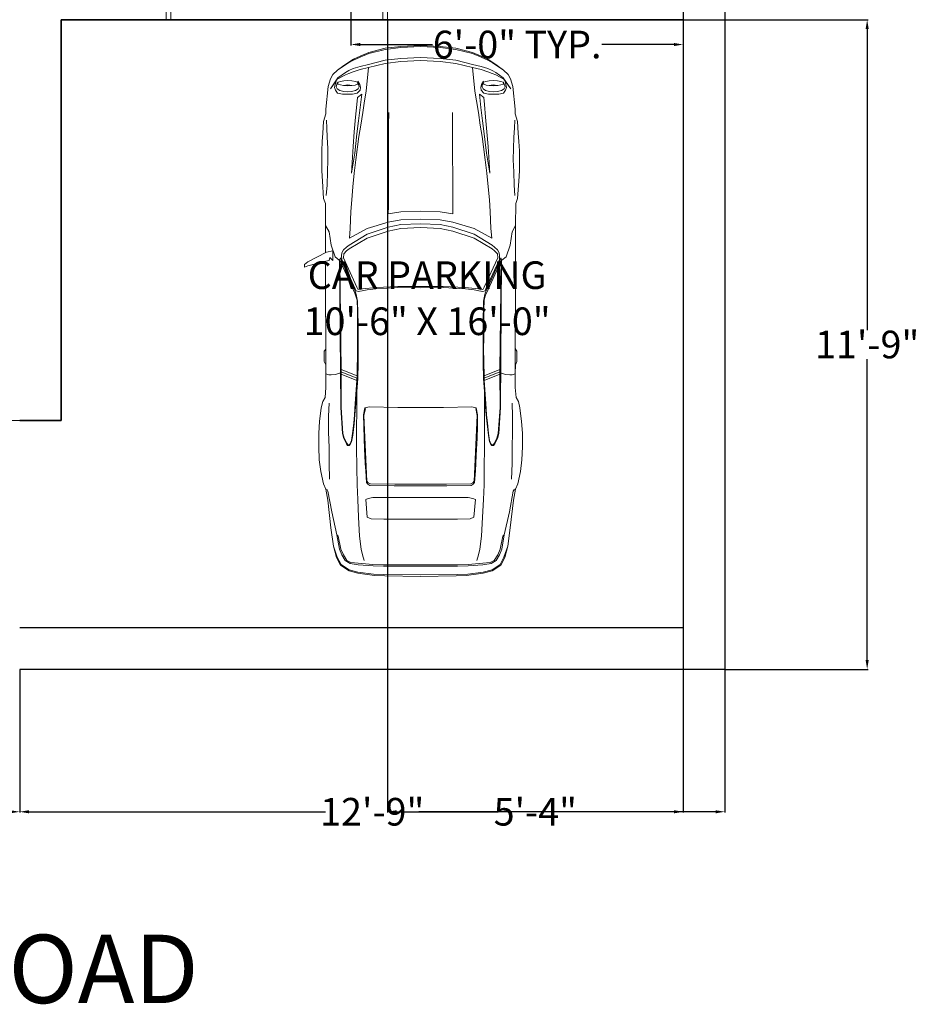
# Model space of a CAD drawing. Units: inches. Extents: x 84 to 590, y 32 to 648.
# Tile 3 of 6: x 340 to 535, y 32 to 245. Entities that reach past the tile are written whole.
import ezdxf

# ---------------------------------------------------------------- set-up
doc = ezdxf.new("R2010")
doc.units = ezdxf.units.IN
doc.header["$MEASUREMENT"] = 0
for name, color, linetype, lineweight in [('A-ANNO-DIMS', 2, 'Continuous', 18), ('A-ANNO-TEXT', 7, 'Continuous', 18), ('A-AREA-IDEN', 7, 'Continuous', 18), ('A-FLOR-STRS', 7, 'Continuous', 18), ('A-GLAZ', 4, 'Continuous', 18), ('A-WALL', 7, 'Continuous', 35), ('C-PARK-VEHI', 8, 'Continuous', 13), ('C-PROP', 7, 'Continuous', 30)]:
    doc.layers.add(name, color=color, linetype=linetype, lineweight=lineweight)
doc.styles.get("Standard").update_dxf_attribs({"font": 'arial.ttf'})
doc.dimstyles.get("Standard").update_dxf_attribs({"dimtxt": 6, "dimasz": 2, "dimexe": 0.18, "dimexo": 0.0625, "dimgap": 0.09, "dimtad": 0, "dimtih": 1, "dimtoh": 1, "dimdec": 0, "dimzin": 0, "dimdsep": 46, "dimlunit": 4, "dimtxsty": 'Standard', "dimcen": 0.09, "dimadec": 0, "dimazin": 0, "dimtfac": 1, "dimtdec": 0, "dimtofl": 0, "dimtmove": 0, "dimatfit": 3, "dimfxl": 1, "dimtolj": 1, "dimtzin": 0, "dimarcsym": 1})

# ---------------------------------------------------------------- blocks, each defined once
blk = doc.blocks.new('WIND')
for p, q in [((-51.89, 1021.98), (-99.89, 1021.98)), ((-99.89, 1021.98), (-99.89, 1012.98)), ((-98.89, 1021.98), (-98.89, 1012.98)), ((-52.89, 1012.98), (-52.89, 1021.98)), ((-51.89, 1012.98), (-51.89, 1021.98)), ((-98.89, 1018.48), (-52.89, 1018.48)), ((-97.89, 1018.48), (-97.89, 1016.48)), ((-97.89, 1017.48), (-53.89, 1017.48)), ((-53.89, 1016.48), (-53.89, 1018.48)), ((-98.89, 1016.48), (-52.89, 1016.48)), ((-99.89, 1012.98), (-51.89, 1012.98))]:
    blk.add_line(p, q)
blk = doc.blocks.new('*D24')
at = {"layer": 'A-ANNO-DIMS', "color": 0, "lineweight": -2, "transparency": 16777216}
for p, q in [((411.91, 254.17), (411.91, 239.77)), ((484.03, 254.17), (484.03, 239.77)), ((413.91, 239.95), (429.58, 239.95)), ((482.03, 239.95), (466.36, 239.95))]:
    blk.add_line(p, q, dxfattribs=at)
at = {"layer": 'A-ANNO-DIMS', "color": 0, "transparency": 16777216}
for points in [[(413.91, 240.28), (413.91, 239.62), (411.91, 239.95)], [(482.03, 240.28), (482.03, 239.62), (484.03, 239.95)]]:
    blk.add_solid(points, dxfattribs=at)
at = {"layer": 'Defpoints', "color": 0, "transparency": 16777216}
for p in [(411.91, 254.23), (484.03, 254.23), (484.03, 239.95)]:
    blk.add_point(p, dxfattribs=at)
at = {"layer": 'A-ANNO-DIMS', "color": 0, "transparency": 16777216, "insert": (447.97, 239.95), "char_height": 6, "attachment_point": 5}
blk.add_mtext('\\A1;6\'-0" TYP.', dxfattribs=at)
blk = doc.blocks.new('*D26')
at = {"layer": 'A-ANNO-DIMS', "color": 0, "lineweight": -2, "transparency": 16777216}
for p, q in [((343.17, 263.92), (343.17, 251.91)), ((359.62, 263.92), (359.62, 251.91)), ((345.17, 252.09), (357.62, 252.09)), ((359.62, 252.09), (361.62, 252.09))]:
    blk.add_line(p, q, dxfattribs=at)
at = {"layer": 'A-ANNO-DIMS', "color": 0, "transparency": 16777216}
for points in [[(345.17, 252.42), (345.17, 251.76), (343.17, 252.09)], [(357.62, 252.42), (357.62, 251.76), (359.62, 252.09)]]:
    blk.add_solid(points, dxfattribs=at)
at = {"layer": 'Defpoints', "color": 0, "transparency": 16777216}
for p in [(343.17, 263.98), (359.62, 263.98), (359.62, 252.09)]:
    blk.add_point(p, dxfattribs=at)
at = {"layer": 'A-ANNO-DIMS', "color": 0, "transparency": 16777216, "insert": (386.71, 252.09), "char_height": 6, "attachment_point": 5}
blk.add_mtext('\\A1;1\'-4 1/2" TYP.', dxfattribs=at)
blk = doc.blocks.new('*D45')
at = {"layer": 'A-ANNO-DIMS', "color": 0, "lineweight": -2, "transparency": 16777216}
for p, q in [((484.09, 245.34), (524.11, 245.34)), ((523.93, 243.34), (523.93, 177.99)), ((523.93, 106.34), (523.93, 171.68)), ((493.09, 104.34), (524.11, 104.34))]:
    blk.add_line(p, q, dxfattribs=at)
at = {"layer": 'A-ANNO-DIMS', "color": 0, "transparency": 16777216}
for points in [[(523.59, 243.34), (524.26, 243.34), (523.93, 245.34)], [(523.59, 106.34), (524.26, 106.34), (523.93, 104.34)]]:
    blk.add_solid(points, dxfattribs=at)
at = {"layer": 'Defpoints', "color": 0, "transparency": 16777216}
for p in [(484.03, 245.34), (493.03, 104.34), (523.93, 104.34)]:
    blk.add_point(p, dxfattribs=at)
at = {"layer": 'A-ANNO-DIMS', "color": 0, "transparency": 16777216, "insert": (523.93, 174.84), "char_height": 6, "attachment_point": 5}
blk.add_mtext('\\A1;11\'-9"', dxfattribs=at)
blk = doc.blocks.new('*D47')
at = {"layer": 'A-ANNO-DIMS', "color": 0, "lineweight": -2, "transparency": 16777216}
for p, q in [((280.03, 104.28), (280.03, 73.26)), ((340.03, 104.28), (340.03, 73.26)), ((282.03, 73.44), (301.96, 73.44)), ((338.03, 73.44), (318.09, 73.44))]:
    blk.add_line(p, q, dxfattribs=at)
at = {"layer": 'A-ANNO-DIMS', "color": 0, "transparency": 16777216}
for points in [[(282.03, 73.77), (282.03, 73.1), (280.03, 73.44)], [(338.03, 73.77), (338.03, 73.1), (340.03, 73.44)]]:
    blk.add_solid(points, dxfattribs=at)
at = {"layer": 'Defpoints', "color": 0, "transparency": 16777216}
for p in [(280.03, 104.34), (340.03, 104.34), (340.03, 73.44)]:
    blk.add_point(p, dxfattribs=at)
at = {"layer": 'A-ANNO-DIMS', "color": 0, "transparency": 16777216, "insert": (310.03, 73.44), "char_height": 6, "attachment_point": 5}
blk.add_mtext('\\A1;5\'-0"', dxfattribs=at)
blk = doc.blocks.new('*D48')
at = {"layer": 'A-ANNO-DIMS', "color": 0, "lineweight": -2, "transparency": 16777216}
for p, q in [((340.03, 104.28), (340.03, 73.26)), ((493.03, 104.28), (493.03, 73.26)), ((342.03, 73.44), (406.42, 73.44)), ((491.03, 73.44), (426.64, 73.44))]:
    blk.add_line(p, q, dxfattribs=at)
at = {"layer": 'A-ANNO-DIMS', "color": 0, "transparency": 16777216}
for points in [[(342.03, 73.77), (342.03, 73.1), (340.03, 73.44)], [(491.03, 73.77), (491.03, 73.1), (493.03, 73.44)]]:
    blk.add_solid(points, dxfattribs=at)
at = {"layer": 'Defpoints', "color": 0, "transparency": 16777216}
for p in [(340.03, 104.34), (493.03, 104.34), (493.03, 73.44)]:
    blk.add_point(p, dxfattribs=at)
at = {"layer": 'A-ANNO-DIMS', "color": 0, "transparency": 16777216, "insert": (416.53, 73.44), "char_height": 6, "attachment_point": 5}
blk.add_mtext('\\A1;12\'-9"', dxfattribs=at)
blk = doc.blocks.new('*D59')
at = {"layer": 'A-ANNO-DIMS', "color": 0, "lineweight": -2, "transparency": 16777216}
for p, q in [((419.82, 245.28), (419.82, 73.26)), ((484.03, 245.28), (484.03, 73.26)), ((421.82, 73.44), (443.86, 73.44)), ((482.03, 73.44), (459.99, 73.44))]:
    blk.add_line(p, q, dxfattribs=at)
at = {"layer": 'A-ANNO-DIMS', "color": 0, "transparency": 16777216}
for points in [[(421.82, 73.77), (421.82, 73.1), (419.82, 73.44)], [(482.03, 73.77), (482.03, 73.1), (484.03, 73.44)]]:
    blk.add_solid(points, dxfattribs=at)
at = {"layer": 'Defpoints', "color": 0, "transparency": 16777216}
for p in [(419.82, 245.34), (484.03, 245.34), (484.03, 73.44)]:
    blk.add_point(p, dxfattribs=at)
at = {"layer": 'A-ANNO-DIMS', "color": 0, "transparency": 16777216, "insert": (451.92, 73.44), "char_height": 6, "attachment_point": 5}
blk.add_mtext('\\A1;5\'-4"', dxfattribs=at)

msp = doc.modelspace()

# ---------------------------------------------------------------- linework, layer by layer
at = {"layer": 'A-FLOR-STRS'}
msp.add_line((280.03, 158.34), (349.03, 158.34), dxfattribs=at)
at = {"layer": 'A-WALL'}
for p, q in [((349.03, 245.34), (484.03, 245.34)), ((349.03, 201.84), (349.03, 245.34)), ((349.03, 158.34), (349.03, 201.84)), ((349.03, 158.34), (340.03, 158.34))]:
    msp.add_line(p, q, dxfattribs=at)
at = {"layer": 'C-PARK-VEHI'}
for p, q in [((422.76, 239.52, -279.43), (419.35, 239.14, -279.43)), ((427.02, 239.73, -279.43), (422.76, 239.52, -279.43)), ((427.02, 239.49, -279.43), (422.76, 239.27, -279.43)), ((427.02, 239.73, -279.43), (427.02, 239.73, -279.43)), ((427.02, 239.73, -279.43), (431.28, 239.52, -279.43)), ((427.02, 239.49, -279.43), (431.28, 239.27, -279.43)), ((431.28, 239.52, -279.43), (434.69, 239.14, -279.43)), ((413.89, 237.44, -279.43), (412.43, 236.8, -279.43)), ((415.76, 238.24, -279.43), (413.89, 237.44, -279.43)), ((415.76, 237.99, -279.43), (413.89, 237.18, -279.43)), ((419.35, 239.14, -279.43), (415.76, 238.24, -279.43)), ((419.35, 238.88, -279.43), (415.76, 237.99, -279.43)), ((422.76, 239.27, -279.43), (419.35, 238.88, -279.43)), ((431.28, 239.27, -279.43), (434.69, 238.88, -279.43)), ((434.69, 239.14, -279.43), (438.27, 238.24, -279.43)), ((434.69, 238.88, -279.43), (438.27, 237.99, -279.43)), ((438.27, 238.24, -279.43), (440.15, 237.44, -279.43)), ((438.27, 237.99, -279.43), (440.15, 237.18, -279.43)), ((440.15, 237.44, -279.43), (441.6, 236.8, -279.43)), ((411.41, 235.99, -279.43), (409.02, 234.37, -279.43)), ((410.39, 235.39, -279.43), (409.02, 234.37, -279.43)), ((412.43, 236.8, -279.43), (410.39, 235.39, -279.43)), ((412.43, 236.54, -279.43), (411.41, 235.99, -279.43)), ((412.42, 234.71, -279.43), (413.88, 235.17, -279.43)), ((413.89, 237.18, -279.43), (412.43, 236.54, -279.43)), ((413.88, 235.17, -279.43), (415.75, 235.65, -279.43)), ((415.75, 235.65, -279.43), (419.33, 236.54, -279.43)), ((419.33, 235.86, -279.43), (415.75, 234.96, -279.43)), ((419.33, 236.54, -279.43), (422.75, 236.93, -279.43)), ((422.75, 236.24, -279.43), (419.33, 235.86, -279.43)), ((422.75, 236.93, -279.43), (427.02, 237.14, -279.43)), ((427.02, 236.45, -279.43), (422.75, 236.24, -279.43)), ((431.29, 236.93, -279.43), (427.02, 237.14, -279.43)), ((427.02, 236.45, -279.43), (431.29, 236.24, -279.43)), ((434.7, 236.54, -279.43), (431.29, 236.93, -279.43)), ((431.29, 236.24, -279.43), (434.7, 235.86, -279.43)), ((438.29, 235.65, -279.43), (434.7, 236.54, -279.43)), ((434.7, 235.86, -279.43), (438.29, 234.96, -279.43)), ((440.16, 235.17, -279.43), (438.29, 235.65, -279.43)), ((440.15, 237.18, -279.43), (441.6, 236.54, -279.43)), ((441.62, 234.71, -279.43), (440.16, 235.17, -279.43)), ((441.6, 236.8, -279.43), (443.64, 235.39, -279.43)), ((441.6, 236.54, -279.43), (442.63, 235.99, -279.43)), ((442.63, 235.99, -279.43), (445.01, 234.37, -279.43)), ((443.64, 235.39, -279.43), (445.01, 234.37, -279.43)), ((408, 233.42, -279.43), (407.48, 232.49, -279.43)), ((409.02, 234.37, -279.43), (408, 233.42, -279.43)), ((410.72, 233.34, -279.43), (408.94, 232.4, -279.43)), ((409.09, 232.75, -279.43), (410.72, 233.86, -279.43)), ((410.72, 233.86, -279.43), (411.48, 234.29, -279.43)), ((411.48, 233.68, -279.43), (410.72, 233.34, -279.43)), ((411.48, 234.29, -279.43), (412.42, 234.71, -279.43)), ((412.42, 234.03, -279.43), (411.48, 233.68, -279.43)), ((413.88, 234.5, -279.43), (412.42, 234.03, -279.43)), ((415.75, 234.96, -279.43), (413.88, 234.5, -279.43)), ((415.75, 234.96, -279.43), (415.21, 229.86, -279.43)), ((438.29, 234.96, -279.43), (440.16, 234.5, -279.43)), ((438.29, 234.96, -279.43), (438.82, 229.86, -279.43)), ((440.16, 234.5, -279.43), (441.62, 234.03, -279.43)), ((442.56, 234.29, -279.43), (441.62, 234.71, -279.43)), ((441.62, 234.03, -279.43), (442.56, 233.68, -279.43)), ((443.32, 233.86, -279.43), (442.56, 234.29, -279.43)), ((442.56, 233.68, -279.43), (443.32, 233.34, -279.43)), ((444.95, 232.75, -279.43), (443.32, 233.86, -279.43)), ((443.32, 233.34, -279.43), (445.1, 232.4, -279.43)), ((445.01, 234.37, -279.43), (446.04, 233.42, -279.43)), ((446.04, 233.42, -279.43), (446.55, 232.49, -279.43)), ((406.97, 230.86, -279.43), (406.46, 225.92, -279.43)), ((407.48, 232.49, -279.43), (406.97, 230.86, -279.43)), ((407.45, 230.34, -279.43), (409.09, 232.75, -279.43)), ((408.94, 232.4, -279.43), (407.45, 230.34, -279.43)), ((408.51, 231.29, -279.43), (408.35, 230.61, -279.43)), ((408.68, 231.98, -279.43), (408.51, 231.29, -279.43)), ((408.69, 230.75, -279.43), (408.94, 231.55, -279.43)), ((409.11, 231.77, -279.43), (408.94, 231.55, -279.43)), ((408.94, 231.55, -279.43), (409.11, 231.35, -279.43)), ((409.61, 231.95, -279.43), (409.11, 231.77, -279.43)), ((409.11, 231.35, -279.43), (409.61, 231.17, -279.43)), ((410.36, 232.07, -279.43), (409.61, 231.95, -279.43)), ((409.61, 231.17, -279.43), (410.29, 231.05, -279.43)), ((410.29, 231.05, -279.43), (411.24, 230.99, -279.43)), ((411.24, 232.11, -279.43), (410.36, 232.07, -279.43)), ((410.36, 231.07, -279.43), (411.24, 231.19, -279.43)), ((412.12, 232.07, -279.43), (411.24, 232.11, -279.43)), ((411.24, 231.19, -279.43), (412.11, 231.04, -279.43)), ((411.24, 230.99, -279.43), (412.12, 231.07, -279.43)), ((412.87, 231.95, -279.43), (412.12, 232.07, -279.43)), ((412.12, 231.07, -279.43), (412.82, 231.15, -279.43)), ((412.82, 231.15, -279.43), (413.33, 231.34, -279.43)), ((413.34, 231.77, -279.43), (412.87, 231.95, -279.43)), ((413.33, 231.34, -279.43), (413.49, 231.55, -279.43)), ((413.49, 231.55, -279.43), (413.34, 231.77, -279.43)), ((413.81, 231.29, -279.43), (413.37, 231.98, -279.43)), ((413.49, 231.55, -279.43), (413.63, 231, -279.43)), ((413.63, 231, -279.43), (413.68, 230.75, -279.43)), ((413.97, 230.61, -279.43), (413.81, 231.29, -279.43)), ((440.07, 230.61, -279.43), (440.23, 231.29, -279.43)), ((440.23, 231.29, -279.43), (440.66, 231.98, -279.43)), ((440.41, 231, -279.43), (440.36, 230.75, -279.43)), ((440.54, 231.55, -279.43), (440.41, 231, -279.43)), ((440.54, 231.55, -279.43), (440.7, 231.77, -279.43)), ((440.71, 231.34, -279.43), (440.54, 231.55, -279.43)), ((440.7, 231.77, -279.43), (441.16, 231.95, -279.43)), ((441.22, 231.15, -279.43), (440.71, 231.34, -279.43)), ((441.16, 231.95, -279.43), (441.92, 232.07, -279.43)), ((441.92, 231.07, -279.43), (441.22, 231.15, -279.43)), ((441.92, 232.07, -279.43), (442.79, 232.11, -279.43)), ((442.79, 230.99, -279.43), (441.92, 231.07, -279.43)), ((442.79, 231.19, -279.43), (441.93, 231.04, -279.43)), ((442.79, 232.11, -279.43), (443.68, 232.07, -279.43)), ((443.68, 231.07, -279.43), (442.79, 231.19, -279.43)), ((443.75, 231.05, -279.43), (442.79, 230.99, -279.43)), ((443.68, 232.07, -279.43), (444.42, 231.95, -279.43)), ((444.42, 231.17, -279.43), (443.75, 231.05, -279.43)), ((444.42, 231.95, -279.43), (444.92, 231.77, -279.43)), ((444.92, 231.35, -279.43), (444.42, 231.17, -279.43)), ((444.92, 231.77, -279.43), (445.1, 231.55, -279.43)), ((445.1, 231.55, -279.43), (444.92, 231.35, -279.43)), ((446.59, 230.34, -279.43), (444.95, 232.75, -279.43)), ((445.1, 232.4, -279.43), (446.59, 230.34, -279.43)), ((445.34, 230.75, -279.43), (445.1, 231.55, -279.43)), ((445.35, 231.98, -279.43), (445.53, 231.29, -279.43)), ((445.53, 231.29, -279.43), (445.69, 230.61, -279.43)), ((446.55, 232.49, -279.43), (447.06, 230.86, -279.43)), ((447.06, 230.86, -279.43), (447.58, 225.92, -279.43)), ((408.35, 230.61, -279.43), (408.56, 230.04, -279.43)), ((408.56, 230.04, -279.43), (409.02, 229.36, -279.43)), ((408.89, 230.32, -279.43), (408.69, 230.75, -279.43)), ((409.49, 229.98, -279.43), (408.89, 230.32, -279.43)), ((409.02, 229.36, -279.43), (410.05, 229.19, -279.43)), ((410.35, 229.75, -279.43), (409.49, 229.98, -279.43)), ((410.05, 229.19, -279.43), (410.9, 229.15, -279.43)), ((411.2, 229.66, -279.43), (410.35, 229.75, -279.43)), ((410.9, 229.15, -279.43), (411.41, 229.15, -279.43)), ((412.05, 229.75, -279.43), (411.2, 229.66, -279.43)), ((411.41, 229.15, -279.43), (412.27, 229.19, -279.43)), ((412.91, 229.98, -279.43), (412.05, 229.75, -279.43)), ((412.27, 229.19, -279.43), (413.29, 229.36, -279.43)), ((413.46, 230.32, -279.43), (412.91, 229.98, -279.43)), ((413.29, 229.36, -279.43), (413.9, 230.04, -279.43)), ((414.24, 229.21, -279.43), (413.3, 228.44, -279.43)), ((413.68, 230.75, -279.43), (413.46, 230.32, -279.43)), ((413.9, 230.04, -279.43), (413.97, 230.61, -279.43)), ((413.93, 226.29, -279.43), (414.24, 229.21, -279.43)), ((415.21, 229.86, -279.43), (414.86, 227.76, -279.43)), ((438.82, 229.86, -279.43), (439.17, 227.76, -279.43)), ((440.1, 226.29, -279.43), (439.8, 229.21, -279.43)), ((439.8, 229.21, -279.43), (440.73, 228.44, -279.43)), ((440.14, 230.04, -279.43), (440.07, 230.61, -279.43)), ((440.74, 229.36, -279.43), (440.14, 230.04, -279.43)), ((440.36, 230.75, -279.43), (440.58, 230.32, -279.43)), ((440.58, 230.32, -279.43), (441.13, 229.98, -279.43)), ((441.77, 229.19, -279.43), (440.74, 229.36, -279.43)), ((441.13, 229.98, -279.43), (441.99, 229.75, -279.43)), ((442.63, 229.15, -279.43), (441.77, 229.19, -279.43)), ((441.99, 229.75, -279.43), (442.84, 229.66, -279.43)), ((443.14, 229.15, -279.43), (442.63, 229.15, -279.43)), ((442.84, 229.66, -279.43), (443.69, 229.75, -279.43)), ((443.99, 229.19, -279.43), (443.14, 229.15, -279.43)), ((443.69, 229.75, -279.43), (444.55, 229.98, -279.43)), ((445.01, 229.36, -279.43), (443.99, 229.19, -279.43)), ((444.55, 229.98, -279.43), (445.14, 230.32, -279.43)), ((445.48, 230.04, -279.43), (445.01, 229.36, -279.43)), ((445.14, 230.32, -279.43), (445.34, 230.75, -279.43)), ((445.69, 230.61, -279.43), (445.48, 230.04, -279.43)), ((413.18, 226.93, -279.43), (412.91, 224.16, -279.43)), ((413.3, 228.44, -279.43), (413.18, 226.93, -279.43)), ((414.86, 227.76, -279.43), (414.47, 225.23, -279.43)), ((439.17, 227.76, -279.43), (439.57, 225.23, -279.43)), ((440.73, 228.44, -279.43), (440.86, 226.93, -279.43)), ((440.86, 226.93, -279.43), (441.13, 224.16, -279.43)), ((406.46, 224.89, -279.43), (405.96, 223.27, -279.43)), ((406.46, 225.92, -279.43), (406.46, 224.89, -279.43)), ((413.56, 223.37, -279.43), (413.93, 226.29, -279.43)), ((414.47, 225.23, -279.43), (414.06, 222.48, -279.43)), ((420.09, 222.48, -279.43), (420.13, 225.23, -279.43)), ((433.94, 222.48, -279.43), (433.91, 225.23, -279.43)), ((439.57, 225.23, -279.43), (439.97, 222.48, -279.43)), ((440.47, 223.37, -279.43), (440.1, 226.29, -279.43)), ((447.58, 225.92, -279.43), (447.58, 224.89, -279.43)), ((447.58, 224.89, -279.43), (448.08, 223.27, -279.43)), ((405.96, 223.27, -279.43), (405.81, 220.71, -279.43)), ((406.58, 223.53, -279.43), (406.66, 221.83, -279.43)), ((412.91, 224.16, -279.43), (412.61, 220.99, -279.43)), ((413.22, 220.54, -279.43), (413.56, 223.37, -279.43)), ((414.06, 222.48, -279.43), (413.65, 220.01, -279.43)), ((420.03, 204.78, -279.43), (420.09, 222.48, -279.43)), ((434, 204.78, -279.43), (433.94, 222.48, -279.43)), ((439.97, 222.48, -279.43), (440.38, 220.01, -279.43)), ((440.81, 220.54, -279.43), (440.47, 223.37, -279.43)), ((441.13, 224.16, -279.43), (441.43, 220.99, -279.43)), ((447.46, 223.53, -279.43), (447.38, 221.83, -279.43)), ((448.08, 223.27, -279.43), (448.23, 220.71, -279.43)), ((405.81, 220.71, -279.43), (405.67, 218.92, -279.43)), ((406.66, 221.83, -279.43), (406.77, 219.86, -279.43)), ((412.61, 220.99, -279.43), (412.39, 217.83, -279.43)), ((412.73, 216.37, -279.43), (413.22, 220.54, -279.43)), ((441.3, 216.37, -279.43), (440.81, 220.54, -279.43)), ((441.43, 220.99, -279.43), (441.65, 217.83, -279.43)), ((447.38, 221.83, -279.43), (447.26, 219.86, -279.43)), ((448.23, 220.71, -279.43), (448.37, 218.92, -279.43)), ((405.67, 218.92, -279.43), (405.59, 216.88, -279.43)), ((406.77, 219.86, -279.43), (406.89, 217.39, -279.43)), ((413.65, 220.01, -279.43), (412.97, 214.92, -279.43)), ((440.38, 220.01, -279.43), (441.07, 214.92, -279.43)), ((447.26, 219.86, -279.43), (447.15, 217.39, -279.43)), ((448.37, 218.92, -279.43), (448.45, 216.88, -279.43)), ((405.59, 216.88, -279.43), (405.59, 214.92, -279.43)), ((406.89, 217.39, -279.43), (406.91, 214.92, -279.43)), ((412.39, 217.83, -279.43), (412, 212.02, -279.43)), ((412, 212.02, -279.43), (412.73, 216.37, -279.43)), ((442.03, 212.02, -279.43), (441.3, 216.37, -279.43)), ((441.65, 217.83, -279.43), (442.03, 212.02, -279.43)), ((447.15, 217.39, -279.43), (447.12, 214.92, -279.43)), ((448.45, 216.88, -279.43), (448.45, 214.92, -279.43)), ((405.59, 214.92, -279.43), (405.59, 212.53, -279.43)), ((406.91, 214.92, -279.43), (406.8, 212.31, -279.43)), ((412.97, 214.92, -279.43), (412.63, 212.02, -279.43)), ((441.07, 214.92, -279.43), (441.41, 212.02, -279.43)), ((447.12, 214.92, -279.43), (447.24, 212.31, -279.43)), ((448.45, 214.92, -279.43), (448.45, 212.53, -279.43)), ((405.59, 212.53, -279.43), (405.73, 210.31, -279.43)), ((406.8, 212.31, -279.43), (406.72, 209.46, -279.43)), ((412.63, 212.02, -279.43), (412.35, 209.03, -279.43)), ((441.41, 212.02, -279.43), (441.69, 209.03, -279.43)), ((447.24, 212.31, -279.43), (447.32, 209.46, -279.43)), ((448.45, 212.53, -279.43), (448.31, 210.31, -279.43)), ((405.73, 210.31, -279.43), (405.96, 206.56, -279.43)), ((406.72, 209.46, -279.43), (406.55, 207.21, -279.43)), ((447.32, 209.46, -279.43), (447.48, 207.21, -279.43)), ((448.31, 210.31, -279.43), (448.08, 206.56, -279.43)), ((412.35, 209.03, -279.43), (412.09, 206.22, -279.43)), ((441.69, 209.03, -279.43), (441.94, 206.22, -279.43)), ((405.96, 206.56, -279.43), (406.36, 205.44, -279.43)), ((406.36, 205.44, -279.43), (406.42, 200.67, -279.43)), ((412.09, 206.22, -279.43), (411.92, 203.74, -279.43)), ((441.94, 206.22, -279.43), (442.12, 203.74, -279.43)), ((447.68, 205.44, -279.43), (447.61, 200.67, -279.43)), ((448.08, 206.56, -279.43), (447.68, 205.44, -279.43)), ((411.92, 203.74, -279.43), (411.76, 200.05, -279.43)), ((420.02, 203.22, -279.43), (420.03, 204.78, -279.43)), ((422.76, 203.64, -279.43), (420.02, 203.22, -279.43)), ((427.02, 203.81, -279.43), (422.76, 203.64, -279.43)), ((427.02, 203.81, -279.43), (431.28, 203.64, -279.43)), ((431.28, 203.64, -279.43), (434.01, 203.22, -279.43)), ((434.01, 203.22, -279.43), (434, 204.78, -279.43)), ((442.12, 203.74, -279.43), (442.28, 200.05, -279.43)), ((415.41, 200.01, -279.43), (420.02, 201.38, -279.43)), ((420.02, 201.38, -279.43), (422.76, 201.89, -279.43)), ((422.76, 200.9, -279.43), (420.02, 200.31, -279.43)), ((422.76, 201.89, -279.43), (427.02, 202.06, -279.43)), ((427.02, 201.07, -279.43), (422.76, 200.9, -279.43)), ((431.28, 201.89, -279.43), (427.02, 202.06, -279.43)), ((427.02, 201.07, -279.43), (431.28, 200.9, -279.43)), ((434.01, 201.38, -279.43), (431.28, 201.89, -279.43)), ((431.28, 200.9, -279.43), (434.01, 200.31, -279.43)), ((438.62, 200.01, -279.43), (434.01, 201.38, -279.43)), ((406.42, 200.67, -279.43), (406.41, 194.76, -279.43)), ((407.15, 199.3, -279.43), (406.42, 200.67, -279.43)), ((407.6, 196.41, -279.43), (407.15, 199.3, -279.43)), ((415.41, 198.77, -279.43), (411.5, 196.41, -279.43)), ((411.76, 200.05, -279.43), (411.58, 197.9, -279.43)), ((411.58, 197.9, -279.43), (415.41, 200.01, -279.43)), ((420.02, 200.31, -279.43), (415.41, 198.77, -279.43)), ((420.02, 199.44, -279.43), (415.41, 197.91, -279.43)), ((422.76, 200.04, -279.43), (420.02, 199.44, -279.43)), ((427.02, 200.21, -279.43), (422.76, 200.04, -279.43)), ((427.02, 200.21, -279.43), (431.28, 200.04, -279.43)), ((431.28, 200.04, -279.43), (434.01, 199.44, -279.43)), ((434.01, 200.31, -279.43), (438.62, 198.77, -279.43)), ((434.01, 199.44, -279.43), (438.62, 197.91, -279.43)), ((442.45, 197.9, -279.43), (438.62, 200.01, -279.43)), ((438.62, 198.77, -279.43), (442.54, 196.41, -279.43)), ((442.28, 200.05, -279.43), (442.45, 197.9, -279.43)), ((446.44, 196.41, -279.43), (446.89, 199.3, -279.43)), ((446.89, 199.3, -279.43), (447.61, 200.67, -279.43)), ((447.61, 200.67, -279.43), (447.62, 194.76, -279.43)), ((415.41, 197.91, -279.43), (411.5, 195.58, -279.43)), ((438.62, 197.91, -279.43), (442.54, 195.58, -279.43)), ((406.63, 194.87, -279.43), (402.54, 192.82, -279.43)), ((408, 195.21, -279.43), (406.63, 194.87, -279.43)), ((408.46, 193.85, -279.43), (407.6, 196.41, -279.43)), ((408, 193.08, -279.43), (408, 195.21, -279.43)), ((409.95, 194.74, -279.43), (409.89, 194.07, -279.43)), ((410.3, 195.38, -279.43), (409.95, 194.74, -279.43)), ((410.35, 194.52, -279.43), (410.29, 193.65, -279.43)), ((410.94, 196, -279.43), (410.3, 195.38, -279.43)), ((410.94, 195.21, -279.43), (410.35, 194.52, -279.43)), ((411.5, 196.41, -279.43), (410.94, 196, -279.43)), ((411.5, 195.58, -279.43), (410.94, 195.21, -279.43)), ((442.54, 196.41, -279.43), (443.09, 196, -279.43)), ((442.54, 195.58, -279.43), (443.09, 195.21, -279.43)), ((443.09, 196, -279.43), (443.73, 195.38, -279.43)), ((443.09, 195.21, -279.43), (443.69, 194.52, -279.43)), ((443.69, 194.52, -279.43), (443.75, 193.65, -279.43)), ((443.73, 195.38, -279.43), (444.08, 194.74, -279.43)), ((444.08, 194.74, -279.43), (444.14, 194.07, -279.43)), ((445.57, 193.85, -279.43), (446.44, 196.41, -279.43)), ((447.61, 192.93, -279.43), (447.62, 194.76, -279.43)), ((402.54, 192.82, -279.43), (401.86, 192.23, -279.43)), ((402.54, 191.89, -279.43), (406.44, 192.93, -279.43)), ((406.42, 192.93, -279.43), (406.47, 168.51, -279.43)), ((406.44, 192.93, -279.43), (407.15, 193.1, -279.43)), ((407.15, 193.1, -279.43), (407.32, 193.76, -279.43)), ((407.32, 193.76, -279.43), (407.73, 193.26, -279.43)), ((407.73, 193.26, -279.43), (408, 193.08, -279.43)), ((409.38, 193.16, -279.43), (408.46, 193.85, -279.43)), ((409.45, 193.16, -279.43), (409.63, 193.64, -279.43)), ((409.7, 161.17, -279.43), (409.45, 193.16, -279.43)), ((409.53, 192.79, -279.43), (409.63, 193.04, -279.43)), ((409.66, 180.69, -279.43), (409.53, 192.79, -279.43)), ((409.63, 193.64, -279.43), (409.85, 192.97, -279.43)), ((409.63, 193.04, -279.43), (409.85, 192.37, -279.43)), ((409.85, 192.97, -279.43), (412.75, 186.62, -279.43)), ((409.85, 192.37, -279.43), (412.75, 186.01, -279.43)), ((409.89, 194.07, -279.43), (409.92, 193.33, -279.43)), ((409.92, 193.33, -279.43), (412.84, 186.91, -279.43)), ((410.29, 193.65, -279.43), (413.19, 187.26, -279.43)), ((443.75, 193.65, -279.43), (440.85, 187.26, -279.43)), ((444.12, 193.33, -279.43), (441.2, 186.91, -279.43)), ((444.19, 192.97, -279.43), (441.29, 186.62, -279.43)), ((444.19, 192.37, -279.43), (441.29, 186.01, -279.43)), ((444.14, 194.07, -279.43), (444.12, 193.33, -279.43)), ((444.41, 193.64, -279.43), (444.19, 192.97, -279.43)), ((444.41, 193.04, -279.43), (444.19, 192.37, -279.43)), ((444.34, 161.17, -279.43), (444.58, 193.16, -279.43)), ((444.37, 180.69, -279.43), (444.5, 192.79, -279.43)), ((444.58, 193.16, -279.43), (444.41, 193.64, -279.43)), ((444.5, 192.79, -279.43), (444.41, 193.04, -279.43)), ((444.65, 193.16, -279.43), (445.57, 193.85, -279.43)), ((447.61, 192.93, -279.43), (447.56, 168.51, -279.43)), ((401.86, 192.23, -279.43), (401.86, 191.63, -279.43)), ((401.86, 191.63, -279.43), (402.54, 191.89, -279.43)), ((412.75, 186.62, -279.43), (412.91, 186.19, -279.43)), ((412.75, 186.01, -279.43), (412.91, 185.58, -279.43)), ((412.84, 186.91, -279.43), (413.04, 186.52, -279.43)), ((412.91, 186.19, -279.43), (413.07, 185.72, -279.43)), ((413.04, 186.52, -279.43), (413.54, 186.36, -279.43)), ((413.19, 187.26, -279.43), (413.42, 186.87, -279.43)), ((413.42, 186.87, -279.43), (413.74, 186.72, -279.43)), ((413.54, 186.36, -279.43), (414.34, 186.52, -279.43)), ((413.74, 186.72, -279.43), (414.43, 186.92, -279.43)), ((414.34, 186.52, -279.43), (415.41, 186.73, -279.43)), ((414.43, 186.92, -279.43), (417.36, 187.22, -279.43)), ((415.41, 186.73, -279.43), (417.3, 186.95, -279.43)), ((417.3, 186.95, -279.43), (422.08, 187.2, -279.43)), ((417.36, 187.22, -279.43), (422.08, 187.41, -279.43)), ((422.08, 187.41, -279.43), (427.02, 187.44, -279.43)), ((422.08, 187.2, -279.43), (427.02, 187.17, -279.43)), ((431.95, 187.41, -279.43), (427.02, 187.44, -279.43)), ((431.95, 187.2, -279.43), (427.02, 187.17, -279.43)), ((436.68, 187.22, -279.43), (431.95, 187.41, -279.43)), ((436.74, 186.95, -279.43), (431.95, 187.2, -279.43)), ((439.6, 186.92, -279.43), (436.68, 187.22, -279.43)), ((438.62, 186.73, -279.43), (436.74, 186.95, -279.43)), ((439.69, 186.52, -279.43), (438.62, 186.73, -279.43)), ((440.3, 186.72, -279.43), (439.6, 186.92, -279.43)), ((440.5, 186.36, -279.43), (439.69, 186.52, -279.43)), ((440.61, 186.87, -279.43), (440.3, 186.72, -279.43)), ((441, 186.52, -279.43), (440.5, 186.36, -279.43)), ((440.85, 187.26, -279.43), (440.61, 186.87, -279.43)), ((441.13, 186.19, -279.43), (440.96, 185.72, -279.43)), ((441.2, 186.91, -279.43), (441, 186.52, -279.43)), ((441.29, 186.62, -279.43), (441.13, 186.19, -279.43)), ((441.29, 186.01, -279.43), (441.13, 185.58, -279.43)), ((412.91, 185.58, -279.43), (413.07, 185.11, -279.43)), ((413.07, 185.72, -279.43), (413.34, 184.24, -279.43)), ((413.07, 185.11, -279.43), (413.23, 184.49, -279.43)), ((413.23, 184.49, -279.43), (413.3, 182.29, -279.43)), ((413.34, 184.24, -279.43), (413.46, 179.34, -279.43)), ((440.7, 184.24, -279.43), (440.58, 179.34, -279.43)), ((440.96, 185.72, -279.43), (440.7, 184.24, -279.43)), ((440.8, 184.49, -279.43), (440.73, 182.29, -279.43)), ((440.96, 185.11, -279.43), (440.8, 184.49, -279.43)), ((441.13, 185.58, -279.43), (440.96, 185.11, -279.43)), ((413.3, 182.29, -279.43), (413.3, 179.35, -279.43)), ((440.73, 182.29, -279.43), (440.73, 179.35, -279.43)), ((409.79, 169.45, -279.43), (409.66, 180.69, -279.43)), ((444.25, 169.45, -279.43), (444.37, 180.69, -279.43)), ((413.3, 179.35, -279.43), (413.32, 176.24, -279.43)), ((413.46, 179.34, -279.43), (413.46, 173.97, -279.43)), ((440.58, 179.34, -279.43), (440.58, 173.97, -279.43)), ((440.73, 179.35, -279.43), (440.72, 176.24, -279.43)), ((413.32, 176.24, -279.43), (413.34, 173.96, -279.43)), ((440.72, 176.24, -279.43), (440.7, 173.96, -279.43)), ((406.45, 173.8, -279.43), (406.11, 173.37, -279.43)), ((406.11, 173.37, -279.43), (406.11, 171.16, -279.43)), ((406.45, 173.97, -279.43), (406.45, 173.8, -279.43)), ((413.34, 173.96, -279.43), (413.25, 168.06, -279.43)), ((413.46, 173.97, -279.43), (413.46, 170.76, -279.43)), ((440.58, 173.97, -279.43), (440.58, 170.76, -279.43)), ((440.7, 173.96, -279.43), (440.79, 168.06, -279.43)), ((447.59, 173.97, -279.43), (447.59, 173.8, -279.43)), ((447.59, 173.8, -279.43), (447.93, 173.37, -279.43)), ((447.93, 173.37, -279.43), (447.93, 171.16, -279.43)), ((406.11, 171.16, -279.43), (406.45, 170.47, -279.43)), ((447.93, 171.16, -279.43), (447.59, 170.47, -279.43)), ((406.45, 170.47, -279.43), (406.45, 169.54, -279.43)), ((409.79, 169.45, -279.43), (413.25, 168.06, -279.43)), ((409.79, 168.6, -279.43), (409.79, 169.45, -279.43)), ((409.79, 168.95, -279.43), (413.22, 167.56, -279.43)), ((413.46, 170.76, -279.43), (413.37, 167.5, -279.43)), ((440.58, 170.76, -279.43), (440.67, 167.5, -279.43)), ((444.25, 169.45, -279.43), (440.79, 168.06, -279.43)), ((444.25, 168.95, -279.43), (440.81, 167.56, -279.43)), ((444.25, 168.6, -279.43), (444.25, 169.45, -279.43)), ((447.59, 170.47, -279.43), (447.59, 169.54, -279.43)), ((406.47, 168.51, -279.43), (406.46, 165.5, -279.43)), ((407.11, 168.26, -279.43), (406.47, 168.51, -279.43)), ((407.64, 168.26, -279.43), (407.11, 168.26, -279.43)), ((408.59, 168.34, -279.43), (407.64, 168.26, -279.43)), ((409.45, 168.6, -279.43), (408.59, 168.34, -279.43)), ((409.79, 168.6, -279.43), (409.45, 168.6, -279.43)), ((409.78, 161.17, -279.43), (409.79, 168.6, -279.43)), ((409.79, 168.44, -279.43), (413.2, 167.07, -279.43)), ((413.2, 167.06, -279.43), (412.86, 162.03, -279.43)), ((413.37, 167.5, -279.43), (413.18, 164.67, -279.43)), ((413.25, 168.06, -279.43), (413.2, 167.06, -279.43)), ((440.67, 167.5, -279.43), (440.86, 164.67, -279.43)), ((440.79, 168.06, -279.43), (440.84, 167.06, -279.43)), ((444.25, 168.44, -279.43), (440.84, 167.07, -279.43)), ((440.84, 167.06, -279.43), (441.17, 162.03, -279.43)), ((444.26, 161.17, -279.43), (444.25, 168.6, -279.43)), ((444.25, 168.6, -279.43), (444.58, 168.6, -279.43)), ((444.58, 168.6, -279.43), (445.45, 168.34, -279.43)), ((445.45, 168.34, -279.43), (446.4, 168.26, -279.43)), ((446.4, 168.26, -279.43), (446.92, 168.26, -279.43)), ((446.92, 168.26, -279.43), (447.56, 168.51, -279.43)), ((447.56, 168.51, -279.43), (447.58, 165.5, -279.43)), ((406.46, 165.5, -279.43), (406.3, 163.31, -279.43)), ((413.18, 164.67, -279.43), (413, 162.03, -279.43)), ((413.18, 164.67, -279.43), (413.15, 152.47, -279.43)), ((440.86, 164.67, -279.43), (441.03, 162.03, -279.43)), ((440.86, 164.67, -279.43), (440.88, 152.47, -279.43)), ((447.58, 165.5, -279.43), (447.74, 163.31, -279.43)), ((405.78, 162.45, -279.43), (405.45, 161.09, -279.43)), ((406.3, 163.31, -279.43), (405.78, 162.45, -279.43)), ((447.74, 163.31, -279.43), (448.25, 162.45, -279.43)), ((448.25, 162.45, -279.43), (448.59, 161.09, -279.43)), ((405.45, 161.09, -279.43), (405.1, 158.11, -279.43)), ((407.16, 162.14, -279.43), (407.07, 159.32, -279.43)), ((410.07, 155.55, -279.43), (409.7, 161.17, -279.43)), ((410.17, 155.53, -279.43), (409.78, 161.17, -279.43)), ((412.86, 162.03, -279.43), (412.69, 159.55, -279.43)), ((413, 162.03, -279.43), (412.75, 159.57, -279.43)), ((414.95, 161.09, -279.43), (414.63, 159.56, -279.43)), ((414.73, 159.45, -279.43), (415.04, 160.97, -279.43)), ((415.92, 161.34, -279.43), (414.95, 161.09, -279.43)), ((422.07, 161.18, -279.43), (415.92, 161.34, -279.43)), ((427.03, 161.17, -279.43), (422.07, 161.18, -279.43)), ((427.01, 161.17, -279.43), (431.97, 161.18, -279.43)), ((431.97, 161.18, -279.43), (438.11, 161.34, -279.43)), ((438.11, 161.34, -279.43), (439.09, 161.09, -279.43)), ((439.31, 159.45, -279.43), (439, 160.97, -279.43)), ((439.09, 161.09, -279.43), (439.4, 159.56, -279.43)), ((441.03, 162.03, -279.43), (441.28, 159.57, -279.43)), ((441.17, 162.03, -279.43), (441.35, 159.55, -279.43)), ((443.86, 155.53, -279.43), (444.26, 161.17, -279.43)), ((443.97, 155.55, -279.43), (444.34, 161.17, -279.43)), ((446.87, 162.14, -279.43), (446.96, 159.32, -279.43)), ((448.59, 161.09, -279.43), (448.94, 158.11, -279.43)), ((407.07, 159.32, -279.43), (407.07, 155.83, -279.43)), ((412.69, 159.55, -279.43), (412.5, 157.87, -279.43)), ((412.75, 159.57, -279.43), (412.59, 157.65, -279.43)), ((414.63, 159.56, -279.43), (414.68, 157.12, -279.43)), ((415.38, 145.21, -279.43), (414.73, 159.45, -279.43)), ((438.66, 145.21, -279.43), (439.31, 159.45, -279.43)), ((439.4, 159.56, -279.43), (439.36, 157.12, -279.43)), ((441.28, 159.57, -279.43), (441.45, 157.65, -279.43)), ((441.35, 159.55, -279.43), (441.53, 157.87, -279.43)), ((446.96, 159.32, -279.43), (446.96, 155.83, -279.43)), ((405.1, 158.11, -279.43), (404.93, 155.63, -279.43)), ((412.5, 157.87, -279.43), (412.27, 155.52, -279.43)), ((412.59, 157.65, -279.43), (412.31, 155.2, -279.43)), ((414.68, 157.12, -279.43), (414.76, 154.46, -279.43)), ((439.36, 157.12, -279.43), (439.28, 154.46, -279.43)), ((441.45, 157.65, -279.43), (441.73, 155.2, -279.43)), ((441.53, 157.87, -279.43), (441.77, 155.52, -279.43)), ((448.94, 158.11, -279.43), (449.1, 155.63, -279.43)), ((404.93, 155.63, -279.43), (404.93, 152.65, -279.43)), ((407.07, 155.83, -279.43), (407.16, 152.5, -279.43)), ((410.34, 154.45, -279.43), (410.07, 155.55, -279.43)), ((410.46, 154.5, -279.43), (410.17, 155.53, -279.43)), ((410.91, 153.29, -279.43), (410.34, 154.45, -279.43)), ((411, 153.4, -279.43), (410.46, 154.5, -279.43)), ((412.02, 154, -279.43), (411.76, 153.26, -279.43)), ((412.27, 155.52, -279.43), (412.02, 154, -279.43)), ((412.31, 155.2, -279.43), (412.06, 153.75, -279.43)), ((414.76, 154.46, -279.43), (414.88, 152.11, -279.43)), ((439.28, 154.46, -279.43), (439.16, 152.11, -279.43)), ((441.73, 155.2, -279.43), (441.97, 153.75, -279.43)), ((441.77, 155.52, -279.43), (442.01, 154, -279.43)), ((442.01, 154, -279.43), (442.28, 153.26, -279.43)), ((443.04, 153.4, -279.43), (443.57, 154.5, -279.43)), ((443.13, 153.29, -279.43), (443.7, 154.45, -279.43)), ((443.57, 154.5, -279.43), (443.86, 155.53, -279.43)), ((443.7, 154.45, -279.43), (443.97, 155.55, -279.43)), ((446.96, 155.83, -279.43), (446.87, 152.5, -279.43)), ((449.1, 155.63, -279.43), (449.1, 152.65, -279.43)), ((404.93, 152.65, -279.43), (405.02, 149.83, -279.43)), ((407.16, 152.5, -279.43), (407.16, 149.05, -279.43)), ((411.17, 152.94, -279.43), (410.91, 153.29, -279.43)), ((411.26, 153.1, -279.43), (411, 153.4, -279.43)), ((411.52, 152.9, -279.43), (411.17, 152.94, -279.43)), ((411.54, 153.09, -279.43), (411.26, 153.1, -279.43)), ((411.76, 153.14, -279.43), (411.52, 152.9, -279.43)), ((411.76, 153.26, -279.43), (411.54, 153.09, -279.43)), ((412.06, 153.75, -279.43), (411.76, 153.14, -279.43)), ((413.15, 152.47, -279.43), (413.2, 148.12, -279.43)), ((414.88, 152.11, -279.43), (414.92, 150.75, -279.43)), ((439.16, 152.11, -279.43), (439.11, 150.75, -279.43)), ((440.88, 152.47, -279.43), (440.84, 148.12, -279.43)), ((441.97, 153.75, -279.43), (442.28, 153.14, -279.43)), ((442.28, 153.26, -279.43), (442.5, 153.09, -279.43)), ((442.28, 153.14, -279.43), (442.51, 152.9, -279.43)), ((442.5, 153.09, -279.43), (442.78, 153.1, -279.43)), ((442.51, 152.9, -279.43), (442.86, 152.94, -279.43)), ((442.78, 153.1, -279.43), (443.04, 153.4, -279.43)), ((442.86, 152.94, -279.43), (443.13, 153.29, -279.43)), ((446.87, 152.5, -279.43), (446.87, 149.05, -279.43)), ((449.1, 152.65, -279.43), (449.02, 149.83, -279.43)), ((405.02, 149.83, -279.43), (405.35, 147.27, -279.43)), ((414.92, 150.75, -279.43), (415.03, 148.99, -279.43)), ((439.11, 150.75, -279.43), (439.01, 148.99, -279.43)), ((449.02, 149.83, -279.43), (448.68, 147.27, -279.43)), ((407.16, 149.05, -279.43), (407.26, 145.59, -279.43)), ((413.2, 148.12, -279.43), (413.25, 144.37, -279.43)), ((415.03, 148.99, -279.43), (415.12, 147.43, -279.43)), ((439.01, 148.99, -279.43), (438.92, 147.43, -279.43)), ((440.84, 148.12, -279.43), (440.79, 144.37, -279.43)), ((446.87, 149.05, -279.43), (446.78, 145.59, -279.43)), ((405.35, 147.27, -279.43), (405.95, 144.63, -279.43)), ((415.12, 147.43, -279.43), (415.28, 144.92, -279.43)), ((438.92, 147.43, -279.43), (438.75, 144.92, -279.43)), ((448.68, 147.27, -279.43), (448.09, 144.63, -279.43)), ((405.95, 144.63, -279.43), (406.44, 143.43, -279.43)), ((406.44, 143.43, -279.43), (406.86, 141.04, -279.43)), ((406.67, 143.43, -279.43), (406.9, 143.01, -279.43)), ((413.25, 144.37, -279.43), (413.39, 141.18, -279.43)), ((415.28, 144.92, -279.43), (415.59, 144.56, -279.43)), ((415.67, 144.85, -279.43), (415.38, 145.21, -279.43)), ((415.59, 144.56, -279.43), (416.04, 144.28, -279.43)), ((416.13, 144.58, -279.43), (415.67, 144.85, -279.43)), ((416.04, 144.28, -279.43), (421.31, 144.18, -279.43)), ((421.4, 144.52, -279.43), (416.13, 144.58, -279.43)), ((421.31, 144.18, -279.43), (427.02, 144.18, -279.43)), ((427.03, 144.52, -279.43), (421.4, 144.52, -279.43)), ((427.01, 144.52, -279.43), (432.64, 144.52, -279.43)), ((432.72, 144.18, -279.43), (427.02, 144.18, -279.43)), ((432.64, 144.52, -279.43), (437.9, 144.58, -279.43)), ((438, 144.28, -279.43), (432.72, 144.18, -279.43)), ((437.9, 144.58, -279.43), (438.37, 144.85, -279.43)), ((438.45, 144.56, -279.43), (438, 144.28, -279.43)), ((438.37, 144.85, -279.43), (438.66, 145.21, -279.43)), ((438.75, 144.92, -279.43), (438.45, 144.56, -279.43)), ((440.79, 144.37, -279.43), (440.65, 141.18, -279.43)), ((447.37, 143.43, -279.43), (447.13, 143.01, -279.43)), ((447.6, 143.43, -279.43), (447.18, 141.04, -279.43)), ((448.09, 144.63, -279.43), (447.6, 143.43, -279.43)), ((406.86, 141.04, -279.43), (407.55, 135.07, -279.43)), ((406.9, 143.01, -279.43), (407.75, 138.52, -279.43)), ((413.39, 141.18, -279.43), (413.56, 137.35, -279.43)), ((415.11, 141.19, -279.43), (415.66, 141.45, -279.43)), ((415.45, 137.34, -279.43), (415.11, 141.19, -279.43)), ((415.66, 141.45, -279.43), (416.69, 141.62, -279.43)), ((416.69, 141.62, -279.43), (421.31, 141.65, -279.43)), ((421.31, 141.65, -279.43), (427.02, 141.65, -279.43)), ((432.72, 141.65, -279.43), (427.02, 141.65, -279.43)), ((437.34, 141.62, -279.43), (432.72, 141.65, -279.43)), ((438.38, 141.45, -279.43), (437.34, 141.62, -279.43)), ((438.93, 141.19, -279.43), (438.38, 141.45, -279.43)), ((438.59, 137.34, -279.43), (438.93, 141.19, -279.43)), ((440.65, 141.18, -279.43), (440.47, 137.35, -279.43)), ((447.13, 143.01, -279.43), (446.28, 138.52, -279.43)), ((447.18, 141.04, -279.43), (446.48, 135.07, -279.43)), ((407.75, 138.52, -279.43), (408.88, 133.53, -279.43)), ((413.56, 137.35, -279.43), (413.79, 133.28, -279.43)), ((416.27, 137.01, -279.43), (415.45, 137.34, -279.43)), ((419.01, 136.92, -279.43), (416.27, 137.01, -279.43)), ((427.02, 136.92, -279.43), (419.01, 136.92, -279.43)), ((427.02, 136.92, -279.43), (435.03, 136.92, -279.43)), ((435.03, 136.92, -279.43), (437.76, 137.01, -279.43)), ((437.76, 137.01, -279.43), (438.59, 137.34, -279.43)), ((440.47, 137.35, -279.43), (440.24, 133.28, -279.43)), ((446.28, 138.52, -279.43), (445.15, 133.53, -279.43)), ((407.55, 135.07, -279.43), (408.09, 131.07, -279.43)), ((446.48, 135.07, -279.43), (445.95, 131.07, -279.43)), ((408.88, 133.53, -279.43), (409.17, 133.28, -279.43)), ((408.88, 133.53, -279.43), (409.41, 130.46, -279.43)), ((409.17, 133.28, -279.43), (409.75, 130.46, -279.43)), ((413.79, 133.28, -279.43), (414.15, 130.46, -279.43)), ((440.24, 133.28, -279.43), (439.88, 130.46, -279.43)), ((444.86, 133.28, -279.43), (444.28, 130.46, -279.43)), ((445.15, 133.53, -279.43), (444.63, 130.46, -279.43)), ((445.15, 133.53, -279.43), (444.86, 133.28, -279.43)), ((408.76, 128.63, -279.43), (408.09, 131.07, -279.43)), ((408.09, 131.07, -279.43), (408.92, 128.68, -279.43)), ((409.41, 130.46, -279.43), (409.93, 129.19, -279.43)), ((409.75, 130.46, -279.43), (410.28, 129.19, -279.43)), ((414.15, 130.46, -279.43), (414.45, 129.19, -279.43)), ((439.88, 130.46, -279.43), (439.59, 129.19, -279.43)), ((444.28, 130.46, -279.43), (443.76, 129.19, -279.43)), ((444.63, 130.46, -279.43), (444.11, 129.19, -279.43)), ((445.95, 131.07, -279.43), (445.12, 128.68, -279.43)), ((445.28, 128.63, -279.43), (445.95, 131.07, -279.43)), ((409.61, 126.97, -279.43), (408.76, 128.63, -279.43)), ((408.92, 128.68, -279.43), (409.78, 127.07, -279.43)), ((409.93, 129.19, -279.43), (410.65, 127.99, -279.43)), ((410.28, 129.19, -279.43), (411.05, 127.99, -279.43)), ((414.45, 129.19, -279.43), (414.79, 127.99, -279.43)), ((439.59, 129.19, -279.43), (439.24, 127.99, -279.43)), ((443.76, 129.19, -279.43), (442.99, 127.99, -279.43)), ((444.11, 129.19, -279.43), (443.39, 127.99, -279.43)), ((445.12, 128.68, -279.43), (444.26, 127.07, -279.43)), ((444.42, 126.97, -279.43), (445.28, 128.63, -279.43)), ((411.5, 125.72, -279.43), (409.61, 126.97, -279.43)), ((409.78, 127.07, -279.43), (411.5, 125.98, -279.43)), ((410.65, 127.99, -279.43), (411.71, 127.35, -279.43)), ((411.05, 127.99, -279.43), (411.92, 127.56, -279.43)), ((411.71, 127.35, -279.43), (413.51, 127.03, -279.43)), ((411.92, 127.56, -279.43), (416.67, 127.08, -279.43)), ((413.51, 127.03, -279.43), (416.7, 126.82, -279.43)), ((416.67, 127.08, -279.43), (418.98, 127.04, -279.43)), ((416.7, 126.82, -279.43), (419, 126.73, -279.43)), ((435.06, 127.04, -279.43), (418.98, 127.04, -279.43)), ((419, 126.73, -279.43), (435.04, 126.73, -279.43)), ((437.33, 126.82, -279.43), (435.04, 126.73, -279.43)), ((437.37, 127.08, -279.43), (435.06, 127.04, -279.43)), ((440.52, 127.03, -279.43), (437.33, 126.82, -279.43)), ((442.12, 127.56, -279.43), (437.37, 127.08, -279.43)), ((442.33, 127.35, -279.43), (440.52, 127.03, -279.43)), ((442.99, 127.99, -279.43), (442.12, 127.56, -279.43)), ((443.39, 127.99, -279.43), (442.33, 127.35, -279.43)), ((444.26, 127.07, -279.43), (442.54, 125.98, -279.43)), ((442.54, 125.72, -279.43), (444.42, 126.97, -279.43)), ((411.5, 125.98, -279.43), (413.43, 125.44, -279.43)), ((413.43, 125.19, -279.43), (411.5, 125.72, -279.43)), ((413.43, 125.44, -279.43), (416.8, 125.02, -279.43)), ((417.05, 124.74, -279.43), (413.43, 125.19, -279.43)), ((416.8, 125.02, -279.43), (419.02, 124.93, -279.43)), ((419.28, 124.65, -279.43), (417.05, 124.74, -279.43)), ((419.02, 124.93, -279.43), (427.02, 124.84, -279.43)), ((427.01, 124.5, -279.43), (419.28, 124.65, -279.43)), ((435.02, 124.93, -279.43), (427.02, 124.84, -279.43)), ((427.03, 124.5, -279.43), (434.76, 124.65, -279.43)), ((434.76, 124.65, -279.43), (436.98, 124.74, -279.43)), ((437.24, 125.02, -279.43), (435.02, 124.93, -279.43)), ((436.98, 124.74, -279.43), (440.6, 125.19, -279.43)), ((440.6, 125.44, -279.43), (437.24, 125.02, -279.43)), ((442.54, 125.98, -279.43), (440.6, 125.44, -279.43)), ((440.6, 125.19, -279.43), (442.54, 125.72, -279.43))]:
    msp.add_line(p, q, dxfattribs=at)
at = {"layer": 'C-PROP'}
for p, q in [((493.03, 608.34), (493.03, 104.34)), ((484.03, 245.34), (484.03, 113.34)), ((484.03, 113.34), (340.03, 113.34)), ((493.03, 104.34), (340.03, 104.34))]:
    msp.add_line(p, q, dxfattribs=at)

# ---------------------------------------------------------------- block references
at = {"layer": 'A-GLAZ'}
msp.add_blockref('WIND', (471.71, -767.64), dxfattribs=at)

# ---------------------------------------------------------------- texts
at = {"layer": 'A-ANNO-TEXT', "insert": (26.34, 46.75), "char_height": 14.8342, "attachment_point": 1}
msp.add_mtext_dynamic_manual_height_columns('\\pxqc;NORTH  ROAD', width=572.5101, gutter_width=74.17, heights=[0], dxfattribs=at)
at = {"layer": 'A-AREA-IDEN', "insert": (350.82, 192.89), "char_height": 6, "attachment_point": 1}
msp.add_mtext_dynamic_manual_height_columns('\\pxqc;CAR PARKING\\P10\'-6" X 16\'-0"', width=155.2362, gutter_width=30, heights=[0], dxfattribs=at)

# ---------------------------------------------------------------- dimensions: what is measured, and where the dimension line sits
at = {"layer": 'A-ANNO-DIMS'}
for base, p1, p2, picture, middle in [((359.6238, 252.0897), (343.1746, 263.9848), (359.6238, 263.9848), '*D26', (386.7084, 252.0897)), ((484.03, 239.95), (411.91, 254.23), (484.03, 254.23), '*D24', (447.97, 239.95))]:
    dim = msp.add_linear_dim(base=base, p1=p1, p2=p2, text='<> TYP.', dimstyle='Standard', override={"dimdec": 1, "dimlfac": 1, "dimrnd": 0, "dimzin": 1, "dimdsep": 46, "dimlunit": 4, "dimfrac": 2}, dxfattribs=at)
    dim.commit()
    dim.dimension.update_dxf_attribs({"geometry": picture, "text_midpoint": middle})
for base, p1, p2, picture, middle in [((484.03, 73.44), (419.82, 245.34), (484.03, 245.34), '*D59', (451.92, 73.44)), ((340.03, 73.44), (280.03, 104.34), (340.03, 104.34), '*D47', (310.03, 73.44)), ((493.03, 73.44), (340.03, 104.34), (493.03, 104.34), '*D48', (416.53, 73.44))]:
    dim = msp.add_linear_dim(base=base, p1=p1, p2=p2, dimstyle='Standard', override={"dimdec": 1, "dimlfac": 1, "dimrnd": 0, "dimzin": 1, "dimdsep": 46, "dimlunit": 4, "dimfrac": 2}, dxfattribs=at)
    dim.commit()
    dim.dimension.update_dxf_attribs({"geometry": picture, "text_midpoint": middle})
dim = msp.add_linear_dim(base=(523.93, 104.34), p1=(484.03, 245.34), p2=(493.03, 104.34), angle=90, dimstyle='Standard', override={"dimdec": 1, "dimlfac": 1, "dimrnd": 0, "dimzin": 1, "dimdsep": 46, "dimlunit": 4, "dimfrac": 2}, dxfattribs=at)
dim.commit()
dim.dimension.update_dxf_attribs({"geometry": '*D45', "text_midpoint": (523.93, 174.84)})

doc.saveas('drawing.dxf')
